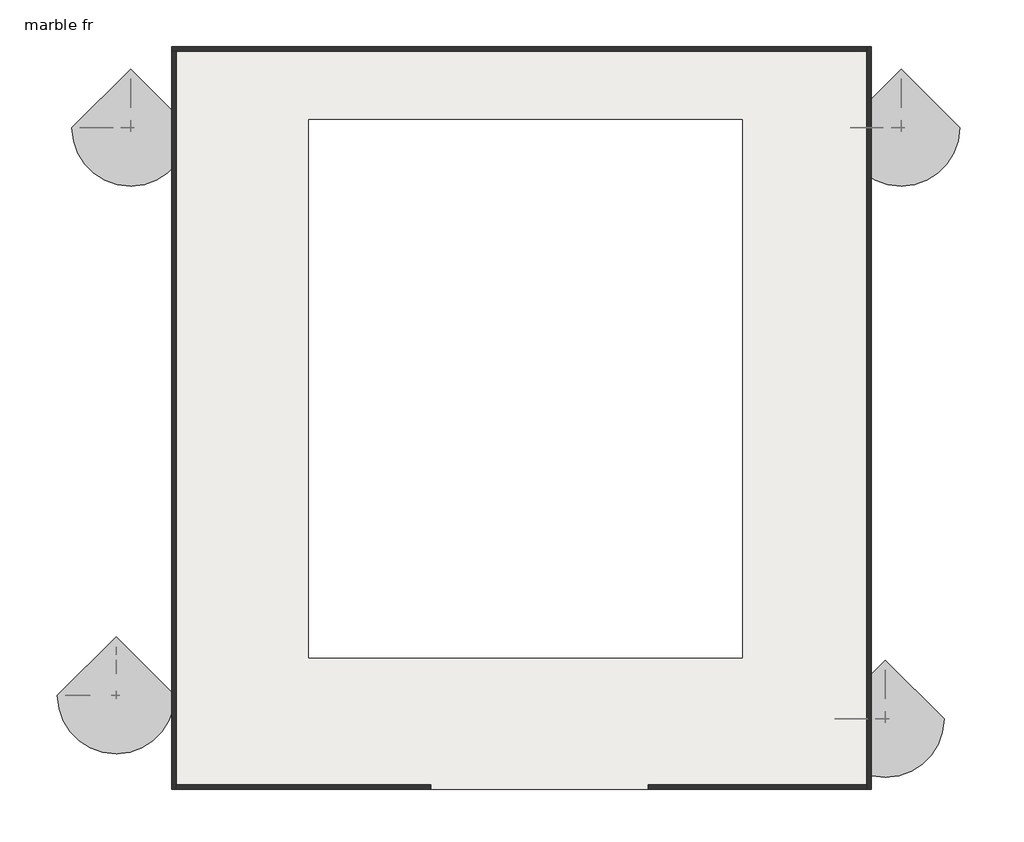
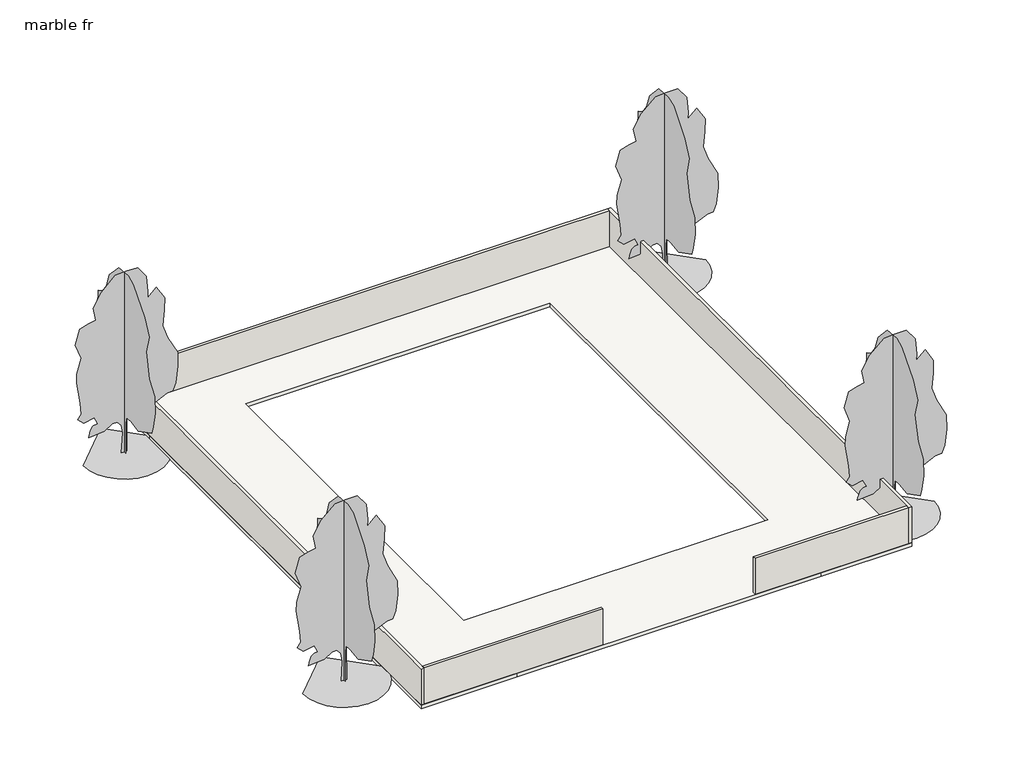
# One storey, incomplete: 5 walls, 4 geographic elements, 1 slab.
"""IFC4 building model written with IfcOpenShell, lengths in millimetres."""

from ifc_helpers import new_model, si_unit, frame, origin, place, context, project, spatial, polyline, outline, extrude, faceted_brep, transform, mapped, element, save
from components import rpc_tree_deciduous_red_ash_25_14781bec

model = new_model("IFC4")

# Units and contexts
model_context = context("Model", 3, world=origin())
ifc_project = project(units=[si_unit("LENGTHUNIT", "METRE", prefix="MILLI")], contexts=[model_context])

# Site, building, storey
site = spatial("IfcSite", under=ifc_project)
building = spatial("IfcBuilding", under=site)
storey = spatial("IfcBuildingStorey", under=building, Name="marble fr", Elevation=-152.4)

# Geographic elements
placement = place(None, origin())
rpc_tree_deciduous_red_ash_25_shape = rpc_tree_deciduous_red_ash_25_14781bec(model_context)
element("IfcGeographicElement", 1, ObjectType="RPC Tree - Deciduous : Red Ash - 25'", at=placement, inside=storey, context=model_context, shape_type="MappedRepresentation", body=[
    mapped(rpc_tree_deciduous_red_ash_25_shape, transform((559.9404734, -8246.7727897, -304.8), x_axis=(1.0, 0.0, 0.0), y_axis=(0.0, 1.0, 0.0), z_axis=(0.0, 0.0, 1.0))),
])
element("IfcGeographicElement", 2, ObjectType="RPC Tree - Deciduous : Red Ash - 25'", at=placement, inside=storey, context=model_context, shape_type="MappedRepresentation", body=[
    mapped(rpc_tree_deciduous_red_ash_25_shape, transform((-21030.0595266, -7586.3727897, -152.4), x_axis=(1.0, 0.0, 0.0), y_axis=(0.0, 1.0, 0.0), z_axis=(0.0, 0.0, 1.0))),
])
element("IfcGeographicElement", 3, ObjectType="RPC Tree - Deciduous : Red Ash - 25'", at=placement, inside=storey, context=model_context, shape_type="MappedRepresentation", body=[
    mapped(rpc_tree_deciduous_red_ash_25_shape, transform((998.7880572, 8352.1272103, -304.8), x_axis=(1.0, 0.0, 0.0), y_axis=(0.0, 1.0, 0.0), z_axis=(0.0, 0.0, 1.0))),
])
element("IfcGeographicElement", 4, ObjectType="RPC Tree - Deciduous : Red Ash - 25'", at=placement, inside=storey, context=model_context, shape_type="MappedRepresentation", body=[
    mapped(rpc_tree_deciduous_red_ash_25_shape, transform((-20623.6595266, 8352.1272103, -304.8), x_axis=(1.0, 0.0, 0.0), y_axis=(0.0, 1.0, 0.0), z_axis=(0.0, 0.0, 1.0))),
])

# Slab
element("IfcSlab", 5, ObjectType="compound marble", at=placement, inside=storey, context=model_context, shape_type="SweptSolid", body=[
    extrude(outline(polyline([(166.2404734, 10629.2155242), (166.2404734, 8580.7272103), (166.2404734, -10224.1844758), (-3455.6771954, -10224.1844758), (-15623.8646954, -10224.1844758), (-19467.9595266, -10224.1844758), (-19467.9595266, 8580.7272103), (-19467.9595266, 10629.2155242), (166.2404734, 10629.2155242)]), holes=[polyline([(-15623.8646954, 8580.7272103), (-15623.8646954, -6532.2727897), (-3455.6771954, -6532.2727897), (-3455.6771954, 8580.7272103), (-15623.8646954, 8580.7272103)])]), frame((0.0, 0.0, -304.8), z_axis=(0.0, 0.0, 1.0), x_axis=(1.0, 0.0, 0.0)), (0.0, 0.0, 1.0), 152.4),
])

# Walls
element("IfcWall", 6, ObjectType="INNER WALL 5\"", at=placement, inside=storey, context=model_context, shape_type="Brep", body=[
    faceted_brep([(-19467.9595266, 10502.2155242, -152.4), (-19340.9595266, 10502.2155242, -152.4), (39.2404734, 10502.2155242, -152.4), (39.2404734, 10502.2155242, 1371.6), (-19340.9595266, 10502.2155242, 1371.6), (-19467.9595266, 10502.2155242, 1371.6), (-19467.9595266, 10629.2155242, -152.4), (-19467.9595266, 10629.2155242, 1371.6), (39.2404734, 10629.2155242, 1371.6), (39.2404734, 10629.2155242, -152.4)], [[[0, 1, 2, 3, 4, 5]], [[6, 7, 8, 9]], [[2, 1, 0, 6, 9]], [[5, 4, 3, 8, 7]], [[0, 5, 7, 6]], [[3, 2, 9, 8]]]),
])
element("IfcWall", 7, ObjectType="INNER WALL 5\"", at=placement, inside=storey, context=model_context, shape_type="Brep", body=[
    faceted_brep([(-19340.9595266, -10224.1844758, -152.4), (-19340.9595266, -10097.1844758, -152.4), (-19340.9595266, 10502.2155242, -152.4), (-19340.9595266, 10502.2155242, 1371.6), (-19340.9595266, -10097.1844758, 1371.6), (-19340.9595266, -10224.1844758, 1371.6), (-19467.9595266, -10224.1844758, -152.4), (-19467.9595266, -10224.1844758, 1371.6), (-19467.9595266, 10502.2155242, 1371.6), (-19467.9595266, 10502.2155242, -152.4)], [[[0, 1, 2, 3, 4, 5]], [[6, 7, 8, 9]], [[2, 1, 0, 6, 9]], [[5, 4, 3, 8, 7]], [[3, 2, 9, 8]], [[0, 5, 7, 6]]]),
])
element("IfcWall", 8, ObjectType="INNER WALL 5\"", at=placement, inside=storey, context=model_context, shape_type="Brep", body=[
    faceted_brep([(39.2404734, 10629.2155242, -152.4), (39.2404734, 10502.2155242, -152.4), (39.2404734, -10097.1844758, -152.4), (39.2404734, -10224.1844758, -152.4), (39.2404734, -10224.1844758, 1371.6), (39.2404734, -10097.1844758, 1371.6), (39.2404734, 10502.2155242, 1371.6), (39.2404734, 10629.2155242, 1371.6), (166.2404734, 10629.2155242, -152.4), (166.2404734, 10629.2155242, 1371.6), (166.2404734, -10224.1844758, 1371.6), (166.2404734, -10224.1844758, -152.4)], [[[0, 1, 2, 3, 4, 5, 6, 7]], [[8, 9, 10, 11]], [[3, 2, 1, 0, 8, 11]], [[7, 6, 5, 4, 10, 9]], [[0, 7, 9, 8]], [[4, 3, 11, 10]]]),
])
element("IfcWall", 9, ObjectType="INNER WALL 5\"", at=placement, inside=storey, context=model_context, shape_type="SweptSolid", body=[
    extrude(outline(polyline([(-12193.2771954, -10224.1844758), (-19340.9595266, -10224.1844758), (-19340.9595266, -10097.1844758), (-12193.2771954, -10097.1844758), (-12193.2771954, -10224.1844758)])), frame((0.0, 0.0, -152.4), z_axis=(0.0, 0.0, 1.0), x_axis=(1.0, 0.0, 0.0)), (0.0, 0.0, 1.0), 1524.0),
])
element("IfcWall", 10, ObjectType="INNER WALL 5\"", at=placement, inside=storey, context=model_context, shape_type="SweptSolid", body=[
    extrude(outline(polyline([(-6097.2771954, -10097.1844758), (39.2404734, -10097.1844758), (39.2404734, -10224.1844758), (-6097.2771954, -10224.1844758), (-6097.2771954, -10097.1844758)])), frame((0.0, 0.0, -152.4), z_axis=(0.0, 0.0, 1.0), x_axis=(1.0, 0.0, 0.0)), (0.0, 0.0, 1.0), 1524.0),
])

save(model, "model.ifc")

# Revit data of these elements
# Type "RPC Tree - Deciduous : Red Ash - 25'"
#   built-in parameter 1005198 = "{2, 15},{22, RPC-8-G3GR-497X-PHW5-6},{1, 0},{1, 0},{2, 37},{1, 8},{5, Color},{1, 0},{1, 0},{3, 0.8},{3, 0.8},{3, 0.8},{1, 8},{7, BBoxMin},{1, 0},{1, 0},{1, 0},{1, 0},{1, 0},{1, 8},{7, BBoxMax},{1, 0},{1, 0},{1, 0},{1, 0},{1, 0},{2, 11},{9, RPCTypeId},{1, 0},{1, 0},{22, RPC-8-G3GR-497X-PHW5-6},{1, 6},{14, RPCPlantHeight},{1, 0},{1, 0},{2, 25},{2, 11},{7, keyword},{1, 0},{1, 0},{78, :Geometry:RPC:Red Ash:red ash:frainus pennsylvanica:frene rouge:deciduous:tree},{2, 11},{8, category},{1, 0},{1, 0},{16, :Trees [General]},{2, 11},{12, LocalizedUID},{1, 0},{1, 0},{7, Red Ash},{2, 14},{6, Height},{1, 0},{1, 0},{2, 25},{1, 2},{16, Cast Reflections},{1, 0},{1, 0},{1, 0},{1, 2},{6, Jitter},{1, 0},{1, 0},{1, 1},{1, 2},{9, Billboard},{1, 0},{1, 0},{1, 0},{1, 2},{12, Cast Shadows},{1, 0},{1, 0},{1, 1},{1, 2},{20, Apply Filter Effects},{1, 0},{1, 0},{1, 0},{2, 11},{28, Apply Filter Effects-Text-FC},{1, 0},{1, 0},{4, None},{2, 11},{20, AdvancedUIDefinition},{1, 0},{1, 0},{0, },{2, 11},{10, AssetLibID},{1, 0},{1, 0},{36, 4D3F6E72-3F99-4203-98E9-AF80B3C7A7A4},{2, 11},{10, BaseSchema},{1, 0},{1, 0},{9, RPCSchema},{2, 11},{12, ExchangeGUID},{1, 0},{1, 0},{0, },{1, 2},{6, Hidden},{1, 0},{1, 0},{1, 0},{1, 4},{11, RPCCategory},{1, 0},{1, 0},{1, 0},{2, 11},{8, RPCImage},{1, 0},{1, 0},{0, },{1, 4},{13, SchemaVersion},{1, 0},{1, 0},{1, 4},{2, 11},{12, UIDefinition},{1, 0},{1, 0},{0, },{2, 11},{6, UIName},{1, 0},{1, 0},{22, RPC-8-G3GR-497X-PHW5-6},{2, 11},{11, VersionGUID},{1, 0},{1, 0},{9, RPCSchema},{2, 11},{9, assettype},{1, 0},{1, 0},{11, RPCGeometry},{2, 11},{11, description},{1, 0},{1, 0},{0, },{2, 11},{9, localname},{1, 0},{1, 0},{3, RPC},{2, 11},{9, localtype},{1, 0},{1, 0},{3, RPC},{1, 4},{8, revision},{1, 0},{1, 0},{1, 1},{2, 11},{9, thumbnail},{1, 0},{1, 0},{0, },{1, 4},{7, version},{1, 0},{1, 0},{1, 1},{1, 2},{20, RPC_Cast Reflections},{1, 0},{1, 0},{1, 1},{1, 2},{10, RPC_Jitter},{1, 0},{1, 0},{1, 1},{1, 2},{13, RPC_Billboard},{1, 0},{1, 0},{1, 0},{1, 2},{16, RPC_Cast Shadows},{1, 0},{1, 0},{1, 1},{21, assetlibrary_base.fbx},{1, 5},"
#   built-in parameter 1005195 = "RPC-8-G3GR-497X-PHW5-6"
#   Type Comments = "Red Maple"
#   Assembly Code = "G2050500"
#   Height = 25' - 0"
#   Default Elevation = 0
# Type "compound marble"
#   Assembly Code = "B1010"
#   Function = 0
#   Layers, outside or top first: 0' - 6" "veranda marble floor" (function 1)
# Type "INNER WALL 5\""
#   Assembly Code = "B2010"
#   Layers, outside or top first: 0' - 5" "OUTER WALL PAINT" (function 1)
# Elements 1, 2, 3, 4 (IfcGeographicElement, "RPC Tree - Deciduous : Red Ash - 25'")
#   Phase Created = New Construction
# Element 5 (IfcSlab, "compound marble")
#   Height Offset From Level = 0' - 0"
#   Phase Created = New Construction
#   Materials on its faces: "veranda marble floor"
# Elements 6, 7, 8, 9, 10 (IfcWall, "INNER WALL 5\"")
#   Top Offset = 0' - 0"
#   Base Offset = 0' - 0"
#   Unconnected Height = 5' - 0"
#   wall height = 5' - 0"
#   Phase Created = New Construction
#   Base Constraint = marble fr
#   Materials on its faces: "OUTER WALL PAINT"
# Materials
#   "veranda marble floor": class "Generic", colour RGB 120 120 120, transparency 0, Cost = 0
#   "OUTER WALL PAINT": class "Generic", colour RGB 120 120 120, transparency 0, Cost = 0
